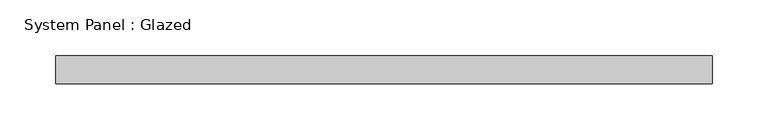
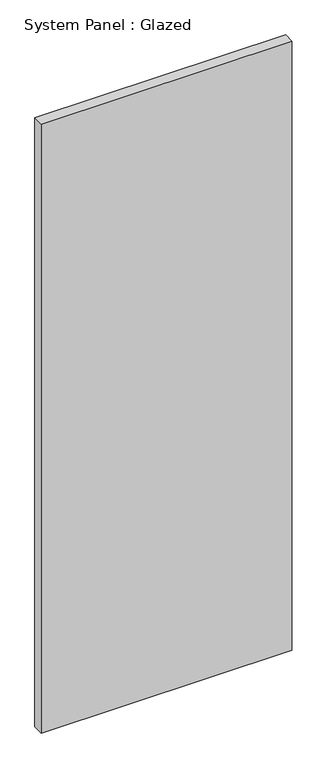
"""IFC4 building model written with IfcOpenShell, lengths in millimetres: plate geometry, System Panel : Glazed."""

from ifc_helpers import new_model, si_unit, origin, origin_with_axes, place, context, project, spatial, polyline, outline, extrude, source, transform, mapped, element, save


def system_panel_glazed_4c12f6d8(model_context):
    return source(origin(), model_context, "Body", "SweptSolid", [
        extrude(outline(polyline([(295.275, 19.05), (-295.275, 19.05), (-295.275, 44.45), (295.275, 44.45), (295.275, 19.05)])), origin_with_axes(), (0.0, 0.0, 1.0), 1517.3056511),
    ])


if __name__ == "__main__":
    model = new_model("IFC4")
    model_context = context("Model", 3, world=origin())
    ifc_project = project(units=[si_unit("LENGTHUNIT", "METRE", prefix="MILLI")], contexts=[model_context])
    site = spatial("IfcSite", under=ifc_project)
    building = spatial("IfcBuilding", under=site)
    placement = place(None, origin())
    system_panel_glazed_shape = system_panel_glazed_4c12f6d8(model_context)
    element("IfcPlate", 1, ObjectType="System Panel : Glazed", at=placement, inside=building, context=model_context, shape_type="MappedRepresentation", body=[
        mapped(system_panel_glazed_shape, transform((0.0, 0.0, 0.0), x_axis=(1.0, 0.0, 0.0), y_axis=(0.0, 1.0, 0.0), z_axis=(0.0, 0.0, 1.0))),
    ])
    save(model, "model.ifc")

# Revit data of these elements
# Type "System Panel : Glazed"
#   Construction Type Id = "GSP4R"
#   Analytic Construction = "1/8 in Pilkington single glazing"
#   Visual Light Transmittance = 0.9
#   Solar Heat Gain Coefficient = 0.86
#   Heat Transfer Coefficient (U) = 1.18115 BTU/(h·ft²·°F)
#   Define Thermal Properties by = 1
# Element 1 (IfcPlate, "System Panel : Glazed")
#   Materials on its faces: "Glass"
# Materials
#   "Glass": class "Glass", colour RGB 0 128 192, transparency 0.75, Description = "Soda Lime Glass", Cost = 0
